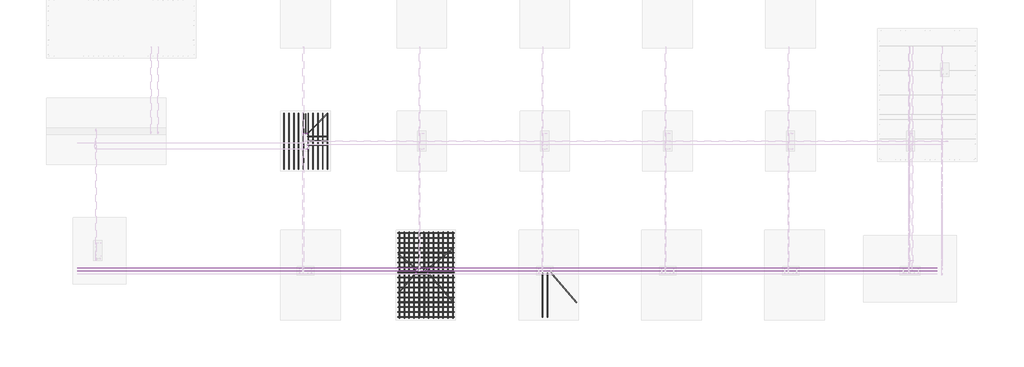
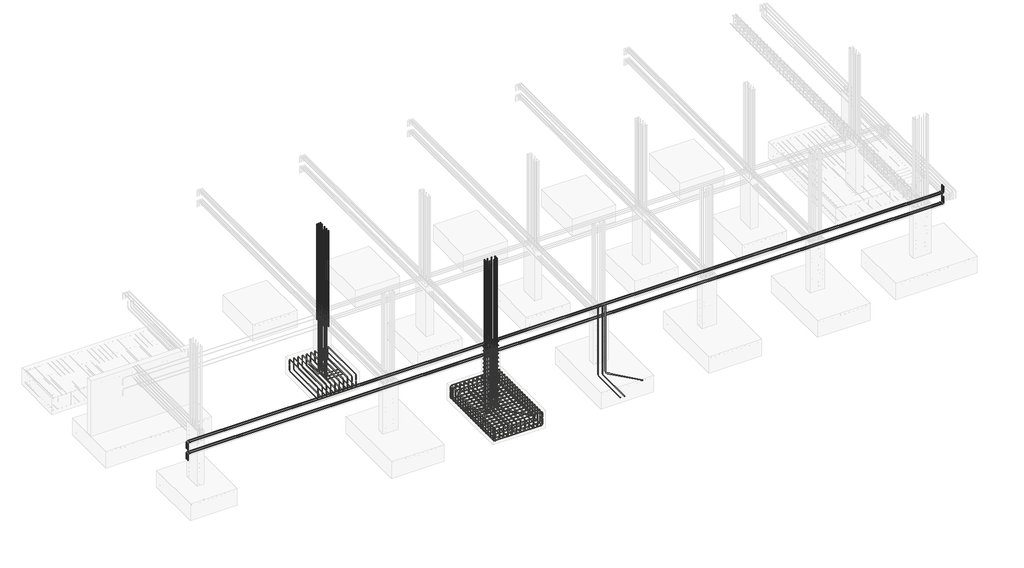
# One storey, part 4 of 18: 38 reinforcing bars.
"""IFC4 building model written with IfcOpenShell, lengths in millimetres."""

from ifc_helpers import new_model, si_unit, point, frame, origin, place, context, project, spatial, polyline, circle_curve, trimmed, segment, composite_curve, source, transform, mapped, element, save
from ifc_brep_helpers import swept_disk

model = new_model("IFC4")

# Units and contexts
model_context = context("Model", 3, world=origin())
ifc_project = project(units=[si_unit("LENGTHUNIT", "METRE", prefix="MILLI")], contexts=[model_context])

# Site, building, storey
site = spatial("IfcSite", under=ifc_project)
building = spatial("IfcBuilding", under=site)
storey = spatial("IfcBuildingStorey", under=building, Elevation=-2000.0)

# Reinforcing bars
placement = place(None, origin())
reinforcing_bar_shape = source(origin(), model_context, "Body", "SolidModel", [
    swept_disk(composite_curve([segment(polyline([(-9318.4091864, -811.9600376, -2322.6684255), (-9318.4091864, -811.9600376, -2470.6684255)]), True, "CONTINUOUS"), segment(trimmed(circle_curve(frame((-9318.4091864, -857.9600376, -2470.6684255), z_axis=(-1.0, 0.0, 0.0), x_axis=(0.0, 46.0, 0.0)), 46.0), [point((-9318.4091864, -811.9600376, -2470.6684255))], [point((-9318.4091864, -857.9600376, -2516.6684255))], True, "CARTESIAN"), True, "CONTINUOUS"), segment(polyline([(-9318.4091864, -857.9600376, -2516.6684255), (-9318.4091864, -2453.9600376, -2516.6684255)]), True, "CONTINUOUS"), segment(trimmed(circle_curve(frame((-9318.4091864, -2453.9600376, -2470.6684255), z_axis=(-1.0, 0.0, 0.0), x_axis=(0.0, 0.0, -46.0)), 46.0), [point((-9318.4091864, -2453.9600376, -2516.6684255))], [point((-9318.4091864, -2499.9600376, -2470.6684255))], True, "CARTESIAN"), True, "CONTINUOUS"), segment(polyline([(-9318.4091864, -2499.9600376, -2470.6684255), (-9318.4091864, -2499.9600376, -2322.6684255)]), True, "CONTINUOUS")], self_intersect=False), 6.0),
])
element("IfcReinforcingBar", 1, at=placement, inside=storey, context=model_context, shape_type="MappedRepresentation", body=[
    mapped(reinforcing_bar_shape, transform((0.0, 0.0, 0.0), x_axis=(1.0, 0.0, 0.0), y_axis=(0.0, 1.0, 0.0), z_axis=(0.0, 0.0, 1.0))),
    mapped(reinforcing_bar_shape, transform((144.8687847, 0.0, 0.0), x_axis=(1.0, 0.0, 0.0), y_axis=(0.0, 1.0, 0.0), z_axis=(0.0, 0.0, 1.0))),
    mapped(reinforcing_bar_shape, transform((289.7375694, 0.0, 0.0), x_axis=(1.0, 0.0, 0.0), y_axis=(0.0, 1.0, 0.0), z_axis=(0.0, 0.0, 1.0))),
    mapped(reinforcing_bar_shape, transform((434.6063541, 0.0, 0.0), x_axis=(1.0, 0.0, 0.0), y_axis=(0.0, 1.0, 0.0), z_axis=(0.0, 0.0, 1.0))),
    mapped(reinforcing_bar_shape, transform((579.4751388, 0.0, 0.0), x_axis=(1.0, 0.0, 0.0), y_axis=(0.0, 1.0, 0.0), z_axis=(0.0, 0.0, 1.0))),
    mapped(reinforcing_bar_shape, transform((724.3439235, 0.0, 0.0), x_axis=(1.0, 0.0, 0.0), y_axis=(0.0, 1.0, 0.0), z_axis=(0.0, 0.0, 1.0))),
    mapped(reinforcing_bar_shape, transform((869.2127082, 0.0, 0.0), x_axis=(1.0, 0.0, 0.0), y_axis=(0.0, 1.0, 0.0), z_axis=(0.0, 0.0, 1.0))),
    mapped(reinforcing_bar_shape, transform((1014.0814929, 0.0, 0.0), x_axis=(1.0, 0.0, 0.0), y_axis=(0.0, 1.0, 0.0), z_axis=(0.0, 0.0, 1.0))),
    mapped(reinforcing_bar_shape, transform((1158.9502776, 0.0, 0.0), x_axis=(1.0, 0.0, 0.0), y_axis=(0.0, 1.0, 0.0), z_axis=(0.0, 0.0, 1.0))),
    mapped(reinforcing_bar_shape, transform((1303.8190623, 0.0, 0.0), x_axis=(1.0, 0.0, 0.0), y_axis=(0.0, 1.0, 0.0), z_axis=(0.0, 0.0, 1.0))),
])
reinforcing_bar_2_shape = source(origin(), model_context, "Body", "SolidModel", [
    swept_disk(composite_curve([segment(polyline([(-8012.6669522, -811.9600376, -2276.6677805), (-8012.6669522, -811.9600376, -2128.6677805)]), True, "CONTINUOUS"), segment(trimmed(circle_curve(frame((-8012.6669522, -857.9600376, -2128.6677805), z_axis=(1.0, 0.0, 0.0), x_axis=(0.0, 46.0, 0.0)), 46.0), [point((-8012.6669522, -811.9600376, -2128.6677805))], [point((-8012.6669522, -857.9600376, -2082.6677805))], True, "CARTESIAN"), True, "CONTINUOUS"), segment(polyline([(-8012.6669522, -857.9600376, -2082.6677805), (-8012.6669522, -2453.9600376, -2082.6677805)]), True, "CONTINUOUS"), segment(trimmed(circle_curve(frame((-8012.6669522, -2453.9600376, -2128.6677805), z_axis=(1.0, 0.0, 0.0), x_axis=(0.0, 0.0, 46.0)), 46.0), [point((-8012.6669522, -2453.9600376, -2082.6677805))], [point((-8012.6669522, -2499.9600376, -2128.6677805))], True, "CARTESIAN"), True, "CONTINUOUS"), segment(polyline([(-8012.6669522, -2499.9600376, -2128.6677805), (-8012.6669522, -2499.9600376, -2276.6677805)]), True, "CONTINUOUS")], self_intersect=False), 6.0),
])
element("IfcReinforcingBar", 2, at=placement, inside=storey, context=model_context, shape_type="MappedRepresentation", body=[
    mapped(reinforcing_bar_2_shape, transform((0.0, 0.0, 0.0), x_axis=(1.0, 0.0, 0.0), y_axis=(0.0, 1.0, 0.0), z_axis=(0.0, 0.0, 1.0))),
    mapped(reinforcing_bar_2_shape, transform((-145.0824705, 0.0, 0.0), x_axis=(1.0, 0.0, 0.0), y_axis=(0.0, 1.0, 0.0), z_axis=(0.0, 0.0, 1.0))),
    mapped(reinforcing_bar_2_shape, transform((-290.1649409, 0.0, 0.0), x_axis=(1.0, 0.0, 0.0), y_axis=(0.0, 1.0, 0.0), z_axis=(0.0, 0.0, 1.0))),
    mapped(reinforcing_bar_2_shape, transform((-435.2474114, 0.0, 0.0), x_axis=(1.0, 0.0, 0.0), y_axis=(0.0, 1.0, 0.0), z_axis=(0.0, 0.0, 1.0))),
    mapped(reinforcing_bar_2_shape, transform((-580.3298819, 0.0, 0.0), x_axis=(1.0, 0.0, 0.0), y_axis=(0.0, 1.0, 0.0), z_axis=(0.0, 0.0, 1.0))),
    mapped(reinforcing_bar_2_shape, transform((-725.4123523, 0.0, 0.0), x_axis=(1.0, 0.0, 0.0), y_axis=(0.0, 1.0, 0.0), z_axis=(0.0, 0.0, 1.0))),
    mapped(reinforcing_bar_2_shape, transform((-870.4948228, 0.0, 0.0), x_axis=(1.0, 0.0, 0.0), y_axis=(0.0, 1.0, 0.0), z_axis=(0.0, 0.0, 1.0))),
    mapped(reinforcing_bar_2_shape, transform((-1015.5772932, 0.0, 0.0), x_axis=(1.0, 0.0, 0.0), y_axis=(0.0, 1.0, 0.0), z_axis=(0.0, 0.0, 1.0))),
    mapped(reinforcing_bar_2_shape, transform((-1160.6597637, 0.0, 0.0), x_axis=(1.0, 0.0, 0.0), y_axis=(0.0, 1.0, 0.0), z_axis=(0.0, 0.0, 1.0))),
    mapped(reinforcing_bar_2_shape, transform((-1305.7422342, 0.0, 0.0), x_axis=(1.0, 0.0, 0.0), y_axis=(0.0, 1.0, 0.0), z_axis=(0.0, 0.0, 1.0))),
])
reinforcing_bar_3_shape = source(origin(), model_context, "Body", "SolidModel", [
    swept_disk(composite_curve([segment(polyline([(-4208.2940057, -4415.5752408, -2300.0), (-4208.2940057, -4415.5752408, -2486.6)]), True, "CONTINUOUS"), segment(trimmed(circle_curve(frame((-4263.7440057, -4415.5752408, -2486.6), z_axis=(0.0, 1.0, 0.0), x_axis=(55.45000000000073, 0.0, 0.0)), 55.45), [point((-4208.2940057, -4415.5752408, -2486.6))], [point((-4263.7440057, -4415.5752408, -2542.05))], True, "CARTESIAN"), True, "CONTINUOUS"), segment(polyline([(-4263.7440057, -4415.5752408, -2542.05), (-5836.9440057, -4415.5752408, -2542.05)]), True, "CONTINUOUS"), segment(trimmed(circle_curve(frame((-5836.9440057, -4415.5752408, -2486.6), z_axis=(0.0, 1.0, 0.0), x_axis=(0.0, 0.0, -55.45000000000027)), 55.45), [point((-5836.9440057, -4415.5752408, -2542.05))], [point((-5892.3940057, -4415.5752408, -2486.6))], True, "CARTESIAN"), True, "CONTINUOUS"), segment(polyline([(-5892.3940057, -4415.5752408, -2486.6), (-5892.3940057, -4415.5752408, -2300.0)]), True, "CONTINUOUS")], self_intersect=False), 7.95),
])
element("IfcReinforcingBar", 3, at=placement, inside=storey, context=model_context, shape_type="MappedRepresentation", body=[
    mapped(reinforcing_bar_3_shape, transform((0.0, 0.0, 0.0), x_axis=(1.0, 0.0, 0.0), y_axis=(0.0, 1.0, 0.0), z_axis=(0.0, 0.0, 1.0))),
    mapped(reinforcing_bar_3_shape, transform((0.0, -148.9809282, 0.0), x_axis=(1.0, 0.0, 0.0), y_axis=(0.0, 1.0, 0.0), z_axis=(0.0, 0.0, 1.0))),
    mapped(reinforcing_bar_3_shape, transform((0.0, -297.9618564, 0.0), x_axis=(1.0, 0.0, 0.0), y_axis=(0.0, 1.0, 0.0), z_axis=(0.0, 0.0, 1.0))),
    mapped(reinforcing_bar_3_shape, transform((0.0, -446.9427846, 0.0), x_axis=(1.0, 0.0, 0.0), y_axis=(0.0, 1.0, 0.0), z_axis=(0.0, 0.0, 1.0))),
    mapped(reinforcing_bar_3_shape, transform((0.0, -595.9237129, 0.0), x_axis=(1.0, 0.0, 0.0), y_axis=(0.0, 1.0, 0.0), z_axis=(0.0, 0.0, 1.0))),
    mapped(reinforcing_bar_3_shape, transform((0.0, -744.9046411, 0.0), x_axis=(1.0, 0.0, 0.0), y_axis=(0.0, 1.0, 0.0), z_axis=(0.0, 0.0, 1.0))),
    mapped(reinforcing_bar_3_shape, transform((0.0, -893.8855693, 0.0), x_axis=(1.0, 0.0, 0.0), y_axis=(0.0, 1.0, 0.0), z_axis=(0.0, 0.0, 1.0))),
    mapped(reinforcing_bar_3_shape, transform((0.0, -1042.8664975, 0.0), x_axis=(1.0, 0.0, 0.0), y_axis=(0.0, 1.0, 0.0), z_axis=(0.0, 0.0, 1.0))),
    mapped(reinforcing_bar_3_shape, transform((0.0, -1191.8474257, 0.0), x_axis=(1.0, 0.0, 0.0), y_axis=(0.0, 1.0, 0.0), z_axis=(0.0, 0.0, 1.0))),
    mapped(reinforcing_bar_3_shape, transform((0.0, -1340.8283539, 0.0), x_axis=(1.0, 0.0, 0.0), y_axis=(0.0, 1.0, 0.0), z_axis=(0.0, 0.0, 1.0))),
    mapped(reinforcing_bar_3_shape, transform((0.0, -1489.8092821, 0.0), x_axis=(1.0, 0.0, 0.0), y_axis=(0.0, 1.0, 0.0), z_axis=(0.0, 0.0, 1.0))),
    mapped(reinforcing_bar_3_shape, transform((0.0, -1638.7902103, 0.0), x_axis=(1.0, 0.0, 0.0), y_axis=(0.0, 1.0, 0.0), z_axis=(0.0, 0.0, 1.0))),
    mapped(reinforcing_bar_3_shape, transform((0.0, -1787.7711386, 0.0), x_axis=(1.0, 0.0, 0.0), y_axis=(0.0, 1.0, 0.0), z_axis=(0.0, 0.0, 1.0))),
    mapped(reinforcing_bar_3_shape, transform((0.0, -1936.7520668, 0.0), x_axis=(1.0, 0.0, 0.0), y_axis=(0.0, 1.0, 0.0), z_axis=(0.0, 0.0, 1.0))),
    mapped(reinforcing_bar_3_shape, transform((0.0, -2085.732995, 0.0), x_axis=(1.0, 0.0, 0.0), y_axis=(0.0, 1.0, 0.0), z_axis=(0.0, 0.0, 1.0))),
    mapped(reinforcing_bar_3_shape, transform((0.0, -2234.7139232, 0.0), x_axis=(1.0, 0.0, 0.0), y_axis=(0.0, 1.0, 0.0), z_axis=(0.0, 0.0, 1.0))),
    mapped(reinforcing_bar_3_shape, transform((0.0, -2383.6948514, 0.0), x_axis=(1.0, 0.0, 0.0), y_axis=(0.0, 1.0, 0.0), z_axis=(0.0, 0.0, 1.0))),
    mapped(reinforcing_bar_3_shape, transform((0.0, -2532.6757796, 0.0), x_axis=(1.0, 0.0, 0.0), y_axis=(0.0, 1.0, 0.0), z_axis=(0.0, 0.0, 1.0))),
])
reinforcing_bar_4_shape = source(origin(), model_context, "Body", "SolidModel", [
    swept_disk(composite_curve([segment(polyline([(-5894.3440057, -4415.5752408, -2250.0), (-5894.3440057, -4415.5752408, -2102.0)]), True, "CONTINUOUS"), segment(trimmed(circle_curve(frame((-5848.3440057, -4415.5752408, -2102.0), z_axis=(0.0, 1.0, 0.0), x_axis=(-46.0, 0.0, 0.0)), 46.0), [point((-5894.3440057, -4415.5752408, -2102.0))], [point((-5848.3440057, -4415.5752408, -2056.0))], True, "CARTESIAN"), True, "CONTINUOUS"), segment(polyline([(-5848.3440057, -4415.5752408, -2056.0), (-4252.3440057, -4415.5752408, -2056.0)]), True, "CONTINUOUS"), segment(trimmed(circle_curve(frame((-4252.3440057, -4415.5752408, -2102.0), z_axis=(0.0, 1.0, 0.0), x_axis=(0.0, 0.0, 46.0)), 46.0), [point((-4252.3440057, -4415.5752408, -2056.0))], [point((-4206.3440057, -4415.5752408, -2102.0))], True, "CARTESIAN"), True, "CONTINUOUS"), segment(polyline([(-4206.3440057, -4415.5752408, -2102.0), (-4206.3440057, -4415.5752408, -2250.0)]), True, "CONTINUOUS")], self_intersect=False), 6.0),
])
element("IfcReinforcingBar", 4, at=placement, inside=storey, context=model_context, shape_type="MappedRepresentation", body=[
    mapped(reinforcing_bar_4_shape, transform((0.0, 0.0, 0.0), x_axis=(1.0, 0.0, 0.0), y_axis=(0.0, 1.0, 0.0), z_axis=(0.0, 0.0, 1.0))),
    mapped(reinforcing_bar_4_shape, transform((0.0, -148.9809282, 0.0), x_axis=(1.0, 0.0, 0.0), y_axis=(0.0, 1.0, 0.0), z_axis=(0.0, 0.0, 1.0))),
    mapped(reinforcing_bar_4_shape, transform((0.0, -297.9618564, 0.0), x_axis=(1.0, 0.0, 0.0), y_axis=(0.0, 1.0, 0.0), z_axis=(0.0, 0.0, 1.0))),
    mapped(reinforcing_bar_4_shape, transform((0.0, -446.9427846, 0.0), x_axis=(1.0, 0.0, 0.0), y_axis=(0.0, 1.0, 0.0), z_axis=(0.0, 0.0, 1.0))),
    mapped(reinforcing_bar_4_shape, transform((0.0, -595.9237129, 0.0), x_axis=(1.0, 0.0, 0.0), y_axis=(0.0, 1.0, 0.0), z_axis=(0.0, 0.0, 1.0))),
    mapped(reinforcing_bar_4_shape, transform((0.0, -744.9046411, 0.0), x_axis=(1.0, 0.0, 0.0), y_axis=(0.0, 1.0, 0.0), z_axis=(0.0, 0.0, 1.0))),
    mapped(reinforcing_bar_4_shape, transform((0.0, -893.8855693, 0.0), x_axis=(1.0, 0.0, 0.0), y_axis=(0.0, 1.0, 0.0), z_axis=(0.0, 0.0, 1.0))),
    mapped(reinforcing_bar_4_shape, transform((0.0, -1042.8664975, 0.0), x_axis=(1.0, 0.0, 0.0), y_axis=(0.0, 1.0, 0.0), z_axis=(0.0, 0.0, 1.0))),
    mapped(reinforcing_bar_4_shape, transform((0.0, -1191.8474257, 0.0), x_axis=(1.0, 0.0, 0.0), y_axis=(0.0, 1.0, 0.0), z_axis=(0.0, 0.0, 1.0))),
    mapped(reinforcing_bar_4_shape, transform((0.0, -1340.8283539, 0.0), x_axis=(1.0, 0.0, 0.0), y_axis=(0.0, 1.0, 0.0), z_axis=(0.0, 0.0, 1.0))),
    mapped(reinforcing_bar_4_shape, transform((0.0, -1489.8092821, 0.0), x_axis=(1.0, 0.0, 0.0), y_axis=(0.0, 1.0, 0.0), z_axis=(0.0, 0.0, 1.0))),
    mapped(reinforcing_bar_4_shape, transform((0.0, -1638.7902103, 0.0), x_axis=(1.0, 0.0, 0.0), y_axis=(0.0, 1.0, 0.0), z_axis=(0.0, 0.0, 1.0))),
    mapped(reinforcing_bar_4_shape, transform((0.0, -1787.7711386, 0.0), x_axis=(1.0, 0.0, 0.0), y_axis=(0.0, 1.0, 0.0), z_axis=(0.0, 0.0, 1.0))),
    mapped(reinforcing_bar_4_shape, transform((0.0, -1936.7520668, 0.0), x_axis=(1.0, 0.0, 0.0), y_axis=(0.0, 1.0, 0.0), z_axis=(0.0, 0.0, 1.0))),
    mapped(reinforcing_bar_4_shape, transform((0.0, -2085.732995, 0.0), x_axis=(1.0, 0.0, 0.0), y_axis=(0.0, 1.0, 0.0), z_axis=(0.0, 0.0, 1.0))),
    mapped(reinforcing_bar_4_shape, transform((0.0, -2234.7139232, 0.0), x_axis=(1.0, 0.0, 0.0), y_axis=(0.0, 1.0, 0.0), z_axis=(0.0, 0.0, 1.0))),
    mapped(reinforcing_bar_4_shape, transform((0.0, -2383.6948514, 0.0), x_axis=(1.0, 0.0, 0.0), y_axis=(0.0, 1.0, 0.0), z_axis=(0.0, 0.0, 1.0))),
    mapped(reinforcing_bar_4_shape, transform((0.0, -2532.6757796, 0.0), x_axis=(1.0, 0.0, 0.0), y_axis=(0.0, 1.0, 0.0), z_axis=(0.0, 0.0, 1.0))),
])
reinforcing_bar_5_shape = source(origin(), model_context, "Body", "SolidModel", [
    swept_disk(composite_curve([segment(polyline([(-5848.1632229, -4392.6797656, -2322.6684255), (-5848.1632229, -4392.6797656, -2470.6684255)]), True, "CONTINUOUS"), segment(trimmed(circle_curve(frame((-5848.1632229, -4438.6797656, -2470.6684255), z_axis=(-1.0, 0.0, 0.0), x_axis=(0.0, 46.0, 0.0)), 46.0), [point((-5848.1632229, -4392.6797656, -2470.6684255))], [point((-5848.1632229, -4438.6797656, -2516.6684255))], True, "CARTESIAN"), True, "CONTINUOUS"), segment(polyline([(-5848.1632229, -4438.6797656, -2516.6684255), (-5848.1632229, -6934.6797656, -2516.6684255)]), True, "CONTINUOUS"), segment(trimmed(circle_curve(frame((-5848.1632229, -6934.6797656, -2470.6684255), z_axis=(-1.0, 0.0, 0.0), x_axis=(0.0, 0.0, -46.0)), 46.0), [point((-5848.1632229, -6934.6797656, -2516.6684255))], [point((-5848.1632229, -6980.6797656, -2470.6684255))], True, "CARTESIAN"), True, "CONTINUOUS"), segment(polyline([(-5848.1632229, -6980.6797656, -2470.6684255), (-5848.1632229, -6980.6797656, -2322.6684255)]), True, "CONTINUOUS")], self_intersect=False), 6.0),
])
element("IfcReinforcingBar", 5, at=placement, inside=storey, context=model_context, shape_type="MappedRepresentation", body=[
    mapped(reinforcing_bar_5_shape, transform((0.0, 0.0, 0.0), x_axis=(1.0, 0.0, 0.0), y_axis=(0.0, 1.0, 0.0), z_axis=(0.0, 0.0, 1.0))),
    mapped(reinforcing_bar_5_shape, transform((145.8017329, 0.0, 0.0), x_axis=(1.0, 0.0, 0.0), y_axis=(0.0, 1.0, 0.0), z_axis=(0.0, 0.0, 1.0))),
    mapped(reinforcing_bar_5_shape, transform((291.6034659, 0.0, 0.0), x_axis=(1.0, 0.0, 0.0), y_axis=(0.0, 1.0, 0.0), z_axis=(0.0, 0.0, 1.0))),
    mapped(reinforcing_bar_5_shape, transform((437.4051988, 0.0, 0.0), x_axis=(1.0, 0.0, 0.0), y_axis=(0.0, 1.0, 0.0), z_axis=(0.0, 0.0, 1.0))),
    mapped(reinforcing_bar_5_shape, transform((583.2069318, 0.0, 0.0), x_axis=(1.0, 0.0, 0.0), y_axis=(0.0, 1.0, 0.0), z_axis=(0.0, 0.0, 1.0))),
    mapped(reinforcing_bar_5_shape, transform((729.0086647, 0.0, 0.0), x_axis=(1.0, 0.0, 0.0), y_axis=(0.0, 1.0, 0.0), z_axis=(0.0, 0.0, 1.0))),
    mapped(reinforcing_bar_5_shape, transform((874.8103976, 0.0, 0.0), x_axis=(1.0, 0.0, 0.0), y_axis=(0.0, 1.0, 0.0), z_axis=(0.0, 0.0, 1.0))),
    mapped(reinforcing_bar_5_shape, transform((1020.6121306, 0.0, 0.0), x_axis=(1.0, 0.0, 0.0), y_axis=(0.0, 1.0, 0.0), z_axis=(0.0, 0.0, 1.0))),
    mapped(reinforcing_bar_5_shape, transform((1166.4138635, 0.0, 0.0), x_axis=(1.0, 0.0, 0.0), y_axis=(0.0, 1.0, 0.0), z_axis=(0.0, 0.0, 1.0))),
    mapped(reinforcing_bar_5_shape, transform((1312.2155965, 0.0, 0.0), x_axis=(1.0, 0.0, 0.0), y_axis=(0.0, 1.0, 0.0), z_axis=(0.0, 0.0, 1.0))),
    mapped(reinforcing_bar_5_shape, transform((1458.0173294, 0.0, 0.0), x_axis=(1.0, 0.0, 0.0), y_axis=(0.0, 1.0, 0.0), z_axis=(0.0, 0.0, 1.0))),
    mapped(reinforcing_bar_5_shape, transform((1603.8190623, 0.0, 0.0), x_axis=(1.0, 0.0, 0.0), y_axis=(0.0, 1.0, 0.0), z_axis=(0.0, 0.0, 1.0))),
])
reinforcing_bar_6_shape = source(origin(), model_context, "Body", "SolidModel", [
    swept_disk(composite_curve([segment(polyline([(-4242.4209887, -4392.6797656, -2276.6677805), (-4242.4209887, -4392.6797656, -2128.6677805)]), True, "CONTINUOUS"), segment(trimmed(circle_curve(frame((-4242.4209887, -4438.6797656, -2128.6677805), z_axis=(1.0, 0.0, 0.0), x_axis=(0.0, 46.0, 0.0)), 46.0), [point((-4242.4209887, -4392.6797656, -2128.6677805))], [point((-4242.4209887, -4438.6797656, -2082.6677805))], True, "CARTESIAN"), True, "CONTINUOUS"), segment(polyline([(-4242.4209887, -4438.6797656, -2082.6677805), (-4242.4209887, -6934.6797656, -2082.6677805)]), True, "CONTINUOUS"), segment(trimmed(circle_curve(frame((-4242.4209887, -6934.6797656, -2128.6677805), z_axis=(1.0, 0.0, 0.0), x_axis=(0.0, 0.0, 46.0)), 46.0), [point((-4242.4209887, -6934.6797656, -2082.6677805))], [point((-4242.4209887, -6980.6797656, -2128.6677805))], True, "CARTESIAN"), True, "CONTINUOUS"), segment(polyline([(-4242.4209887, -6980.6797656, -2128.6677805), (-4242.4209887, -6980.6797656, -2276.6677805)]), True, "CONTINUOUS")], self_intersect=False), 6.0),
])
element("IfcReinforcingBar", 6, at=placement, inside=storey, context=model_context, shape_type="MappedRepresentation", body=[
    mapped(reinforcing_bar_6_shape, transform((0.0, 0.0, 0.0), x_axis=(1.0, 0.0, 0.0), y_axis=(0.0, 1.0, 0.0), z_axis=(0.0, 0.0, 1.0))),
    mapped(reinforcing_bar_6_shape, transform((-145.9765667, 0.0, 0.0), x_axis=(1.0, 0.0, 0.0), y_axis=(0.0, 1.0, 0.0), z_axis=(0.0, 0.0, 1.0))),
    mapped(reinforcing_bar_6_shape, transform((-291.9531335, 0.0, 0.0), x_axis=(1.0, 0.0, 0.0), y_axis=(0.0, 1.0, 0.0), z_axis=(0.0, 0.0, 1.0))),
    mapped(reinforcing_bar_6_shape, transform((-437.9297002, 0.0, 0.0), x_axis=(1.0, 0.0, 0.0), y_axis=(0.0, 1.0, 0.0), z_axis=(0.0, 0.0, 1.0))),
    mapped(reinforcing_bar_6_shape, transform((-583.906267, 0.0, 0.0), x_axis=(1.0, 0.0, 0.0), y_axis=(0.0, 1.0, 0.0), z_axis=(0.0, 0.0, 1.0))),
    mapped(reinforcing_bar_6_shape, transform((-729.8828337, 0.0, 0.0), x_axis=(1.0, 0.0, 0.0), y_axis=(0.0, 1.0, 0.0), z_axis=(0.0, 0.0, 1.0))),
    mapped(reinforcing_bar_6_shape, transform((-875.8594005, 0.0, 0.0), x_axis=(1.0, 0.0, 0.0), y_axis=(0.0, 1.0, 0.0), z_axis=(0.0, 0.0, 1.0))),
    mapped(reinforcing_bar_6_shape, transform((-1021.8359672, 0.0, 0.0), x_axis=(1.0, 0.0, 0.0), y_axis=(0.0, 1.0, 0.0), z_axis=(0.0, 0.0, 1.0))),
    mapped(reinforcing_bar_6_shape, transform((-1167.8125339, 0.0, 0.0), x_axis=(1.0, 0.0, 0.0), y_axis=(0.0, 1.0, 0.0), z_axis=(0.0, 0.0, 1.0))),
    mapped(reinforcing_bar_6_shape, transform((-1313.7891007, 0.0, 0.0), x_axis=(1.0, 0.0, 0.0), y_axis=(0.0, 1.0, 0.0), z_axis=(0.0, 0.0, 1.0))),
    mapped(reinforcing_bar_6_shape, transform((-1459.7656674, 0.0, 0.0), x_axis=(1.0, 0.0, 0.0), y_axis=(0.0, 1.0, 0.0), z_axis=(0.0, 0.0, 1.0))),
    mapped(reinforcing_bar_6_shape, transform((-1605.7422342, 0.0, 0.0), x_axis=(1.0, 0.0, 0.0), y_axis=(0.0, 1.0, 0.0), z_axis=(0.0, 0.0, 1.0))),
])
element("IfcReinforcingBar", 7, at=placement, inside=storey, context=model_context, shape_type="SolidModel", body=[
    swept_disk(composite_curve([segment(polyline([(-520.063822, -6507.758358, -2480.0), (-1248.148149, -5670.1931504, -2480.0)]), True, "CONTINUOUS"), segment(trimmed(circle_curve(frame((-1248.148149, -5670.1931504, -2412.5), z_axis=(0.7547095802227678, 0.6560590289905122, 0.0), x_axis=(0.0, 0.0, -67.5)), 67.5), [point((-1248.148149, -5670.1931504, -2480.0))], [point((-1292.4321335, -5619.2502537, -2412.5))], True, "CARTESIAN"), True, "CONTINUOUS"), segment(polyline([(-1292.4321335, -5619.2502537, -2412.5), (-1292.4321335, -5619.2502537, -20.0)]), True, "CONTINUOUS")], self_intersect=False), 10.0),
])
reinforcing_bar_7_shape = source(origin(), model_context, "Body", "SolidModel", [
    swept_disk(composite_curve([segment(polyline([(-1543.6420643, -6948.2510204, -2480.0), (-1543.6420643, -5673.717598, -2480.0)]), True, "CONTINUOUS"), segment(trimmed(circle_curve(frame((-1543.6420643, -5673.717598, -2434.0), z_axis=(1.0, 0.0, 0.0), x_axis=(0.0, 0.0, -46.0)), 46.0), [point((-1543.6420643, -5673.717598, -2480.0))], [point((-1543.6420643, -5627.717598, -2434.0))], True, "CARTESIAN"), True, "CONTINUOUS"), segment(polyline([(-1543.6420643, -5627.717598, -2434.0), (-1543.6420643, -5627.717598, -30.0)]), True, "CONTINUOUS")], self_intersect=False), 6.0),
])
element("IfcReinforcingBar", 8, at=placement, inside=storey, context=model_context, shape_type="MappedRepresentation", body=[
    mapped(reinforcing_bar_7_shape, transform((0.0, 0.0, 0.0), x_axis=(1.0, 0.0, 0.0), y_axis=(0.0, 1.0, 0.0), z_axis=(0.0, 0.0, 1.0))),
    mapped(reinforcing_bar_7_shape, transform((144.9594019, 0.0, 0.0), x_axis=(1.0, 0.0, 0.0), y_axis=(0.0, 1.0, 0.0), z_axis=(0.0, 0.0, 1.0))),
])
reinforcing_bar_8_shape = source(origin(), model_context, "Body", "SolidModel", [
    swept_disk(composite_curve([segment(polyline([(-5060.4315175, -5535.5091206, -34.0), (-5004.0960659, -5479.1736689, -34.0)]), True, "CONTINUOUS"), segment(trimmed(circle_curve(frame((-4983.5899692, -5499.6797656, -34.0), z_axis=(0.0, 0.0, -1.0), x_axis=(-20.506096699999944, 20.506096699999944, 0.0)), 29.0), [point((-5004.0960659, -5479.1736689, -34.0))], [point((-4954.5899692, -5499.6797656, -34.0))], True, "CARTESIAN"), True, "CONTINUOUS"), segment(polyline([(-4954.5899692, -5499.6797656, -34.0), (-4954.5899692, -5623.6797656, -34.0)]), True, "CONTINUOUS"), segment(trimmed(circle_curve(frame((-4983.5899692, -5623.6797656, -34.0), z_axis=(0.0, 0.0, -1.0), x_axis=(29.0, 0.0, 0.0)), 29.0), [point((-4954.5899692, -5623.6797656, -34.0))], [point((-4983.5899692, -5652.6797656, -34.0))], True, "CARTESIAN"), True, "CONTINUOUS"), segment(polyline([(-4983.5899692, -5652.6797656, -34.0), (-5357.5899692, -5652.6797656, -34.0)]), True, "CONTINUOUS"), segment(trimmed(circle_curve(frame((-5357.5899692, -5623.707741, -32.7265044), z_axis=(0.0, 0.043913640913297095, -0.9990353307775146), x_axis=(0.0, -28.972024599999713, -1.2734955999999968)), 29.0), [point((-5357.5899692, -5652.6797656, -34.0))], [point((-5386.5899692, -5623.707741, -32.7265044))], True, "CARTESIAN"), True, "CONTINUOUS"), segment(polyline([(-5386.5899692, -5623.707741, -32.7265044), (-5386.5899692, -5499.6517902, -27.2734956)]), True, "CONTINUOUS"), segment(trimmed(circle_curve(frame((-5357.5899692, -5499.6517902, -27.2734956), z_axis=(0.0, 0.043913640913297095, -0.9990353307775146), x_axis=(-29.0, 0.0, 0.0)), 29.0), [point((-5386.5899692, -5499.6517902, -27.2734956))], [point((-5357.5899692, -5470.6797656, -26.0))], True, "CARTESIAN"), True, "CONTINUOUS"), segment(polyline([(-5357.5899692, -5470.6797656, -26.0), (-4983.5899692, -5470.6797656, -26.0)]), True, "CONTINUOUS"), segment(trimmed(circle_curve(frame((-4983.5899692, -5499.6797656, -26.0), z_axis=(0.0, 0.0, -1.0), x_axis=(0.0, 29.0, 0.0)), 29.0), [point((-4983.5899692, -5470.6797656, -26.0))], [point((-4963.0838726, -5520.1858622, -26.0))], True, "CARTESIAN"), True, "CONTINUOUS"), segment(polyline([(-4963.0838726, -5520.1858622, -26.0), (-5019.4193242, -5576.5213139, -26.0)]), True, "CONTINUOUS")], self_intersect=False), 4.0),
])
element("IfcReinforcingBar", 9, at=placement, inside=storey, context=model_context, shape_type="MappedRepresentation", body=[
    mapped(reinforcing_bar_8_shape, transform((0.0, 0.0, 0.0), x_axis=(1.0, 0.0, 0.0), y_axis=(0.0, 1.0, 0.0), z_axis=(0.0, 0.0, 1.0))),
    mapped(reinforcing_bar_8_shape, transform((0.0, 0.0, -148.6153846), x_axis=(1.0, 0.0, 0.0), y_axis=(0.0, 1.0, 0.0), z_axis=(0.0, 0.0, 1.0))),
    mapped(reinforcing_bar_8_shape, transform((0.0, 0.0, -297.2307692), x_axis=(1.0, 0.0, 0.0), y_axis=(0.0, 1.0, 0.0), z_axis=(0.0, 0.0, 1.0))),
    mapped(reinforcing_bar_8_shape, transform((0.0, 0.0, -445.8461538), x_axis=(1.0, 0.0, 0.0), y_axis=(0.0, 1.0, 0.0), z_axis=(0.0, 0.0, 1.0))),
    mapped(reinforcing_bar_8_shape, transform((0.0, 0.0, -594.4615385), x_axis=(1.0, 0.0, 0.0), y_axis=(0.0, 1.0, 0.0), z_axis=(0.0, 0.0, 1.0))),
    mapped(reinforcing_bar_8_shape, transform((0.0, 0.0, -743.0769231), x_axis=(1.0, 0.0, 0.0), y_axis=(0.0, 1.0, 0.0), z_axis=(0.0, 0.0, 1.0))),
    mapped(reinforcing_bar_8_shape, transform((0.0, 0.0, -891.6923077), x_axis=(1.0, 0.0, 0.0), y_axis=(0.0, 1.0, 0.0), z_axis=(0.0, 0.0, 1.0))),
    mapped(reinforcing_bar_8_shape, transform((0.0, 0.0, -1040.3076923), x_axis=(1.0, 0.0, 0.0), y_axis=(0.0, 1.0, 0.0), z_axis=(0.0, 0.0, 1.0))),
    mapped(reinforcing_bar_8_shape, transform((0.0, 0.0, -1188.9230769), x_axis=(1.0, 0.0, 0.0), y_axis=(0.0, 1.0, 0.0), z_axis=(0.0, 0.0, 1.0))),
    mapped(reinforcing_bar_8_shape, transform((0.0, 0.0, -1337.5384615), x_axis=(1.0, 0.0, 0.0), y_axis=(0.0, 1.0, 0.0), z_axis=(0.0, 0.0, 1.0))),
    mapped(reinforcing_bar_8_shape, transform((0.0, 0.0, -1486.1538462), x_axis=(1.0, 0.0, 0.0), y_axis=(0.0, 1.0, 0.0), z_axis=(0.0, 0.0, 1.0))),
    mapped(reinforcing_bar_8_shape, transform((0.0, 0.0, -1634.7692308), x_axis=(1.0, 0.0, 0.0), y_axis=(0.0, 1.0, 0.0), z_axis=(0.0, 0.0, 1.0))),
    mapped(reinforcing_bar_8_shape, transform((0.0, 0.0, -1783.3846154), x_axis=(1.0, 0.0, 0.0), y_axis=(0.0, 1.0, 0.0), z_axis=(0.0, 0.0, 1.0))),
    mapped(reinforcing_bar_8_shape, transform((0.0, 0.0, -1932.0), x_axis=(1.0, 0.0, 0.0), y_axis=(0.0, 1.0, 0.0), z_axis=(0.0, 0.0, 1.0))),
])
element("IfcReinforcingBar", 10, at=placement, inside=storey, context=model_context, shape_type="SolidModel", body=[
    swept_disk(composite_curve([segment(polyline([(-5873.6233428, -5063.6864072, -2480.0), (-5400.4558049, -5460.7211138, -2480.0)]), True, "CONTINUOUS"), segment(trimmed(circle_curve(frame((-5400.4558049, -5460.7211138, -2412.5), z_axis=(-0.6427876096865429, -0.766044443118975, 0.0), x_axis=(0.0, 0.0, -67.5)), 67.5), [point((-5400.4558049, -5460.7211138, -2480.0))], [point((-5348.747805, -5504.1092774, -2412.5))], True, "CARTESIAN"), True, "CONTINUOUS"), segment(polyline([(-5348.747805, -5504.1092774, -2412.5), (-5348.747805, -5504.1092774, -20.0)]), True, "CONTINUOUS")], self_intersect=False), 10.0),
])
element("IfcReinforcingBar", 11, at=placement, inside=storey, context=model_context, shape_type="SolidModel", body=[
    swept_disk(composite_curve([segment(polyline([(-5877.6576621, -5559.3632831, -2480.0), (-5405.107931, -5559.3632831, -2480.0)]), True, "CONTINUOUS"), segment(trimmed(circle_curve(frame((-5405.107931, -5559.3632831, -2434.0), z_axis=(0.0, -1.0, 0.0), x_axis=(0.0, 0.0, -46.0)), 46.0), [point((-5405.107931, -5559.3632831, -2480.0))], [point((-5359.107931, -5559.3632831, -2434.0))], True, "CARTESIAN"), True, "CONTINUOUS"), segment(polyline([(-5359.107931, -5559.3632831, -2434.0), (-5359.107931, -5559.3632831, -30.0)]), True, "CONTINUOUS")], self_intersect=False), 6.0),
])
element("IfcReinforcingBar", 12, at=placement, inside=storey, context=model_context, shape_type="SolidModel", body=[
    swept_disk(composite_curve([segment(polyline([(-4227.0646685, -4861.8897199, -2480.0), (-4940.7241336, -5460.7211138, -2480.0)]), True, "CONTINUOUS"), segment(trimmed(circle_curve(frame((-4940.7241336, -5460.7211138, -2412.5), z_axis=(-0.6427876096865429, 0.766044443118975, 0.0), x_axis=(0.0, 0.0, -67.5)), 67.5), [point((-4940.7241336, -5460.7211138, -2480.0))], [point((-4992.4321335, -5504.1092774, -2412.5))], True, "CARTESIAN"), True, "CONTINUOUS"), segment(polyline([(-4992.4321335, -5504.1092774, -2412.5), (-4992.4321335, -5504.1092774, -20.0)]), True, "CONTINUOUS")], self_intersect=False), 10.0),
])
element("IfcReinforcingBar", 13, at=placement, inside=storey, context=model_context, shape_type="SolidModel", body=[
    swept_disk(composite_curve([segment(polyline([(-5880.6241894, -6231.1040429, -2480.0), (-5393.0317894, -5670.1931504, -2480.0)]), True, "CONTINUOUS"), segment(trimmed(circle_curve(frame((-5393.0317894, -5670.1931504, -2412.5), z_axis=(0.7547095802227678, -0.6560590289905122, 0.0), x_axis=(0.0, 0.0, -67.5)), 67.5), [point((-5393.0317894, -5670.1931504, -2480.0))], [point((-5348.747805, -5619.2502537, -2412.5))], True, "CARTESIAN"), True, "CONTINUOUS"), segment(polyline([(-5348.747805, -5619.2502537, -2412.5), (-5348.747805, -5619.2502537, -20.0)]), True, "CONTINUOUS")], self_intersect=False), 10.0),
])
element("IfcReinforcingBar", 14, at=placement, inside=storey, context=model_context, shape_type="SolidModel", body=[
    swept_disk(composite_curve([segment(polyline([(-4220.063822, -6507.758358, -2480.0), (-4948.148149, -5670.1931504, -2480.0)]), True, "CONTINUOUS"), segment(trimmed(circle_curve(frame((-4948.148149, -5670.1931504, -2412.5), z_axis=(0.7547095802227678, 0.6560590289905122, 0.0), x_axis=(0.0, 0.0, -67.5)), 67.5), [point((-4948.148149, -5670.1931504, -2480.0))], [point((-4992.4321335, -5619.2502537, -2412.5))], True, "CARTESIAN"), True, "CONTINUOUS"), segment(polyline([(-4992.4321335, -5619.2502537, -2412.5), (-4992.4321335, -5619.2502537, -20.0)]), True, "CONTINUOUS")], self_intersect=False), 10.0),
])
element("IfcReinforcingBar", 15, at=placement, inside=storey, context=model_context, shape_type="SolidModel", body=[
    swept_disk(composite_curve([segment(polyline([(-4223.0303493, -5559.3632831, -2480.0), (-4936.0720074, -5559.3632831, -2480.0)]), True, "CONTINUOUS"), segment(trimmed(circle_curve(frame((-4936.0720074, -5559.3632831, -2434.0), z_axis=(0.0, 1.0, 0.0), x_axis=(0.0, 0.0, -46.0)), 46.0), [point((-4936.0720074, -5559.3632831, -2480.0))], [point((-4982.0720074, -5559.3632831, -2434.0))], True, "CARTESIAN"), True, "CONTINUOUS"), segment(polyline([(-4982.0720074, -5559.3632831, -2434.0), (-4982.0720074, -5559.3632831, -30.0)]), True, "CONTINUOUS")], self_intersect=False), 6.0),
])
reinforcing_bar_9_shape = source(origin(), model_context, "Body", "SolidModel", [
    swept_disk(composite_curve([segment(polyline([(-5243.6420643, -6948.2510204, -2480.0), (-5243.6420643, -5673.717598, -2480.0)]), True, "CONTINUOUS"), segment(trimmed(circle_curve(frame((-5243.6420643, -5673.717598, -2434.0), z_axis=(1.0, 0.0, 0.0), x_axis=(0.0, 0.0, -46.0)), 46.0), [point((-5243.6420643, -5673.717598, -2480.0))], [point((-5243.6420643, -5627.717598, -2434.0))], True, "CARTESIAN"), True, "CONTINUOUS"), segment(polyline([(-5243.6420643, -5627.717598, -2434.0), (-5243.6420643, -5627.717598, -30.0)]), True, "CONTINUOUS")], self_intersect=False), 6.0),
])
element("IfcReinforcingBar", 16, at=placement, inside=storey, context=model_context, shape_type="MappedRepresentation", body=[
    mapped(reinforcing_bar_9_shape, transform((0.0, 0.0, 0.0), x_axis=(1.0, 0.0, 0.0), y_axis=(0.0, 1.0, 0.0), z_axis=(0.0, 0.0, 1.0))),
    mapped(reinforcing_bar_9_shape, transform((144.9594019, 0.0, 0.0), x_axis=(1.0, 0.0, 0.0), y_axis=(0.0, 1.0, 0.0), z_axis=(0.0, 0.0, 1.0))),
])
reinforcing_bar_10_shape = source(origin(), model_context, "Body", "SolidModel", [
    swept_disk(composite_curve([segment(polyline([(-5243.6420643, -4416.634351, -2480.0), (-5243.6420643, -5449.6419331, -2480.0)]), True, "CONTINUOUS"), segment(trimmed(circle_curve(frame((-5243.6420643, -5449.6419331, -2434.0), z_axis=(-1.0, 0.0, 0.0), x_axis=(0.0, 0.0, -46.0)), 46.0), [point((-5243.6420643, -5449.6419331, -2480.0))], [point((-5243.6420643, -5495.6419331, -2434.0))], True, "CARTESIAN"), True, "CONTINUOUS"), segment(polyline([(-5243.6420643, -5495.6419331, -2434.0), (-5243.6420643, -5495.6419331, -30.0)]), True, "CONTINUOUS")], self_intersect=False), 6.0),
])
element("IfcReinforcingBar", 17, at=placement, inside=storey, context=model_context, shape_type="MappedRepresentation", body=[
    mapped(reinforcing_bar_10_shape, transform((0.0, 0.0, 0.0), x_axis=(1.0, 0.0, 0.0), y_axis=(0.0, 1.0, 0.0), z_axis=(0.0, 0.0, 1.0))),
    mapped(reinforcing_bar_10_shape, transform((144.9594019, 0.0, 0.0), x_axis=(1.0, 0.0, 0.0), y_axis=(0.0, 1.0, 0.0), z_axis=(0.0, 0.0, 1.0))),
])
element("IfcReinforcingBar", 18, at=placement, inside=storey, context=model_context, shape_type="SolidModel", body=[
    swept_disk(composite_curve([segment(polyline([(-8671.037887, -1418.4824597, -30.0), (-8671.037887, -1418.4824597, -2440.6)]), True, "CONTINUOUS"), segment(trimmed(circle_curve(frame((-8671.037887, -1372.4824597, -2440.6), z_axis=(1.0, 0.0, 0.0), x_axis=(0.0, -46.0, 0.0)), 46.0), [point((-8671.037887, -1418.4824597, -2440.6))], [point((-8671.037887, -1372.4824597, -2486.6))], True, "CARTESIAN"), True, "CONTINUOUS"), segment(polyline([(-8671.037887, -1372.4824597, -2486.6), (-8671.037887, -834.8555128, -2486.6)]), True, "CONTINUOUS")], self_intersect=False), 6.0),
])
reinforcing_bar_11_shape = source(origin(), model_context, "Body", "SolidModel", [
    swept_disk(composite_curve([segment(polyline([(-8606.6833135, -1776.5422299, -30.0), (-8606.6833135, -1776.5422299, -2436.6982733)]), True, "CONTINUOUS"), segment(trimmed(circle_curve(frame((-8560.6833135, -1776.5422299, -2436.6982733), z_axis=(0.0, -1.0, 0.0), x_axis=(-46.0, 0.0, 0.0)), 46.0), [point((-8606.6833135, -1776.5422299, -2436.6982733))], [point((-8560.6833135, -1776.5422299, -2482.6982733))], True, "CARTESIAN"), True, "CONTINUOUS"), segment(polyline([(-8560.6833135, -1776.5422299, -2482.6982733), (-8021.3501017, -1776.5422299, -2482.6982733)]), True, "CONTINUOUS")], self_intersect=False), 6.0),
])
element("IfcReinforcingBar", 19, at=placement, inside=storey, context=model_context, shape_type="MappedRepresentation", body=[
    mapped(reinforcing_bar_11_shape, transform((0.0, 0.0, 0.0), x_axis=(1.0, 0.0, 0.0), y_axis=(0.0, 1.0, 0.0), z_axis=(0.0, 0.0, 1.0))),
    mapped(reinforcing_bar_11_shape, transform((0.0, 134.2724138, 0.0), x_axis=(1.0, 0.0, 0.0), y_axis=(0.0, 1.0, 0.0), z_axis=(0.0, 0.0, 1.0))),
    mapped(reinforcing_bar_11_shape, transform((0.0, 268.5448277, 0.0), x_axis=(1.0, 0.0, 0.0), y_axis=(0.0, 1.0, 0.0), z_axis=(0.0, 0.0, 1.0))),
])
element("IfcReinforcingBar", 20, at=placement, inside=storey, context=model_context, shape_type="SolidModel", body=[
    swept_disk(composite_curve([segment(polyline([(-8612.8440331, -1423.0839981, -30.0), (-8612.8440331, -1423.0839981, -2431.15)]), True, "CONTINUOUS"), segment(trimmed(circle_curve(frame((-8573.634962, -1383.874927, -2431.15), z_axis=(0.7071067811865501, -0.707106781186545, 0.0), x_axis=(-39.209071100000074, -39.209071099999846, 0.0)), 55.45), [point((-8612.8440331, -1423.0839981, -2431.15))], [point((-8573.634962, -1383.874927, -2486.6))], True, "CARTESIAN"), True, "CONTINUOUS"), segment(polyline([(-8573.634962, -1383.874927, -2486.6), (-8027.7896484, -838.0296134, -2486.6)]), True, "CONTINUOUS")], self_intersect=False), 7.95),
])
reinforcing_bar_12_shape = source(origin(), model_context, "Body", "SolidModel", [
    swept_disk(composite_curve([segment(polyline([(-15532.6790491, -5561.6797656, -300.2534207), (-15532.6790491, -5561.6797656, -113.6534207)]), True, "CONTINUOUS"), segment(trimmed(circle_curve(frame((-15477.2290491, -5561.6797656, -113.6534207), z_axis=(0.0, 1.0, 0.0), x_axis=(-55.44999999999891, 0.0, 0.0)), 55.45), [point((-15532.6790491, -5561.6797656, -113.6534207))], [point((-15477.2290491, -5561.6797656, -58.2034207))], True, "CARTESIAN"), True, "CONTINUOUS"), segment(polyline([(-15477.2290491, -5561.6797656, -58.2034207), (10261.1848807, -5561.6797656, -58.2034207)]), True, "CONTINUOUS"), segment(trimmed(circle_curve(frame((10261.1848807, -5561.6797656, -2.7534207), z_axis=(0.0, -1.0, 0.0), x_axis=(0.0, 0.0, -55.45)), 55.45), [point((10261.1848807, -5561.6797656, -58.2034207))], [point((10316.6348807, -5561.6797656, -2.7534207))], True, "CARTESIAN"), True, "CONTINUOUS"), segment(polyline([(10316.6348807, -5561.6797656, -2.7534207), (10316.6348807, -5561.6797656, 183.8465793)]), True, "CONTINUOUS")], self_intersect=False), 7.95),
])
element("IfcReinforcingBar", 21, at=placement, inside=storey, context=model_context, shape_type="MappedRepresentation", body=[
    mapped(reinforcing_bar_12_shape, transform((0.0, 0.0, 0.0), x_axis=(1.0, 0.0, 0.0), y_axis=(0.0, 1.0, 0.0), z_axis=(0.0, 0.0, 1.0))),
    mapped(reinforcing_bar_12_shape, transform((0.0, 0.0, -384.9941108), x_axis=(1.0, 0.0, 0.0), y_axis=(0.0, 1.0, 0.0), z_axis=(0.0, 0.0, 1.0))),
])
reinforcing_bar_13_shape = source(origin(), model_context, "Body", "SolidModel", [
    swept_disk(composite_curve([segment(polyline([(-15532.6790491, -5469.1797656, -303.2034207), (-15532.6790491, -5469.1797656, -116.6034207)]), True, "CONTINUOUS"), segment(trimmed(circle_curve(frame((-15477.2290491, -5469.1797656, -116.6034207), z_axis=(0.0, 1.0, 0.0), x_axis=(-55.44999999999891, 0.0, 0.0)), 55.45), [point((-15532.6790491, -5469.1797656, -116.6034207))], [point((-15477.2290491, -5469.1797656, -61.1534207))], True, "CARTESIAN"), True, "CONTINUOUS"), segment(polyline([(-15477.2290491, -5469.1797656, -61.1534207), (10261.1848807, -5469.1797656, -61.1534207)]), True, "CONTINUOUS"), segment(trimmed(circle_curve(frame((10261.1848807, -5469.1797656, -5.7034207), z_axis=(0.0, -1.0, 0.0), x_axis=(0.0, 0.0, -55.449999999999996)), 55.45), [point((10261.1848807, -5469.1797656, -61.1534207))], [point((10316.6348807, -5469.1797656, -5.7034207))], True, "CARTESIAN"), True, "CONTINUOUS"), segment(polyline([(10316.6348807, -5469.1797656, -5.7034207), (10316.6348807, -5469.1797656, 180.8965793)]), True, "CONTINUOUS")], self_intersect=False), 7.95),
])
element("IfcReinforcingBar", 22, at=placement, inside=storey, context=model_context, shape_type="MappedRepresentation", body=[
    mapped(reinforcing_bar_13_shape, transform((0.0, 0.0, 0.0), x_axis=(1.0, 0.0, 0.0), y_axis=(0.0, 1.0, 0.0), z_axis=(0.0, 0.0, 1.0))),
    mapped(reinforcing_bar_13_shape, transform((0.0, 0.0, -384.9941108), x_axis=(1.0, 0.0, 0.0), y_axis=(0.0, 1.0, 0.0), z_axis=(0.0, 0.0, 1.0))),
])
element("IfcReinforcingBar", 23, at=placement, inside=storey, context=model_context, shape_type="SolidModel", body=[
    swept_disk(composite_curve([segment(polyline([(-8728.3359054, -1423.0839981, 2970.0), (-8728.3359054, -1423.0839981, -486.6)]), True, "CONTINUOUS")], self_intersect=False), 7.95),
])
element("IfcReinforcingBar", 24, at=placement, inside=storey, context=model_context, shape_type="SolidModel", body=[
    swept_disk(composite_curve([segment(polyline([(-8671.037887, -1418.4824597, 2970.0), (-8671.037887, -1418.4824597, -486.6)]), True, "CONTINUOUS")], self_intersect=False), 6.0),
])
reinforcing_bar_14_shape = source(origin(), model_context, "Body", "SolidModel", [
    swept_disk(composite_curve([segment(polyline([(-8734.496625, -1776.5422299, 2970.0), (-8734.496625, -1776.5422299, -482.6982733)]), True, "CONTINUOUS")], self_intersect=False), 6.0),
])
element("IfcReinforcingBar", 25, at=placement, inside=storey, context=model_context, shape_type="MappedRepresentation", body=[
    mapped(reinforcing_bar_14_shape, transform((0.0, 0.0, 0.0), x_axis=(1.0, 0.0, 0.0), y_axis=(0.0, 1.0, 0.0), z_axis=(0.0, 0.0, 1.0))),
    mapped(reinforcing_bar_14_shape, transform((0.0, 134.2724138, 0.0), x_axis=(1.0, 0.0, 0.0), y_axis=(0.0, 1.0, 0.0), z_axis=(0.0, 0.0, 1.0))),
    mapped(reinforcing_bar_14_shape, transform((0.0, 268.5448277, 0.0), x_axis=(1.0, 0.0, 0.0), y_axis=(0.0, 1.0, 0.0), z_axis=(0.0, 0.0, 1.0))),
])
reinforcing_bar_15_shape = source(origin(), model_context, "Body", "SolidModel", [
    swept_disk(composite_curve([segment(polyline([(-8606.6833135, -1776.5422299, 2970.0), (-8606.6833135, -1776.5422299, -482.6982733)]), True, "CONTINUOUS")], self_intersect=False), 6.0),
])
element("IfcReinforcingBar", 26, at=placement, inside=storey, context=model_context, shape_type="MappedRepresentation", body=[
    mapped(reinforcing_bar_15_shape, transform((0.0, 0.0, 0.0), x_axis=(1.0, 0.0, 0.0), y_axis=(0.0, 1.0, 0.0), z_axis=(0.0, 0.0, 1.0))),
    mapped(reinforcing_bar_15_shape, transform((0.0, 134.2724138, 0.0), x_axis=(1.0, 0.0, 0.0), y_axis=(0.0, 1.0, 0.0), z_axis=(0.0, 0.0, 1.0))),
    mapped(reinforcing_bar_15_shape, transform((0.0, 268.5448277, 0.0), x_axis=(1.0, 0.0, 0.0), y_axis=(0.0, 1.0, 0.0), z_axis=(0.0, 0.0, 1.0))),
])
element("IfcReinforcingBar", 27, at=placement, inside=storey, context=model_context, shape_type="SolidModel", body=[
    swept_disk(composite_curve([segment(polyline([(-8671.037887, -1896.3217695, 2970.0), (-8671.037887, -1896.3217695, -486.6)]), True, "CONTINUOUS")], self_intersect=False), 6.0),
])
element("IfcReinforcingBar", 28, at=placement, inside=storey, context=model_context, shape_type="SolidModel", body=[
    swept_disk(composite_curve([segment(polyline([(-8612.8440331, -1423.0839981, 2970.0), (-8612.8440331, -1423.0839981, -486.6)]), True, "CONTINUOUS")], self_intersect=False), 7.95),
])
element("IfcReinforcingBar", 29, at=placement, inside=storey, context=model_context, shape_type="SolidModel", body=[
    swept_disk(composite_curve([segment(polyline([(-8728.3359054, -1891.7202311, 2970.0), (-8728.3359054, -1891.7202311, -486.6)]), True, "CONTINUOUS")], self_intersect=False), 7.95),
])
element("IfcReinforcingBar", 30, at=placement, inside=storey, context=model_context, shape_type="SolidModel", body=[
    swept_disk(composite_curve([segment(polyline([(-8612.8440331, -1891.7202311, 2970.0), (-8612.8440331, -1891.7202311, -486.6)]), True, "CONTINUOUS")], self_intersect=False), 7.95),
])
element("IfcReinforcingBar", 31, at=placement, inside=storey, context=model_context, shape_type="SolidModel", body=[
    swept_disk(composite_curve([segment(polyline([(-5359.1470109, -5560.0856321, -480.0), (-5359.1470109, -5560.0856321, 2970.0)]), True, "CONTINUOUS")], self_intersect=False), 6.0),
])
element("IfcReinforcingBar", 32, at=placement, inside=storey, context=model_context, shape_type="SolidModel", body=[
    swept_disk(composite_curve([segment(polyline([(-5002.4712133, -5504.8316264, -480.0), (-5002.4712133, -5504.8316264, 2970.0)]), True, "CONTINUOUS")], self_intersect=False), 10.0),
])
element("IfcReinforcingBar", 33, at=placement, inside=storey, context=model_context, shape_type="SolidModel", body=[
    swept_disk(composite_curve([segment(polyline([(-5358.7868848, -5619.9726027, -480.0), (-5358.7868848, -5619.9726027, 2970.0)]), True, "CONTINUOUS")], self_intersect=False), 10.0),
])
element("IfcReinforcingBar", 34, at=placement, inside=storey, context=model_context, shape_type="SolidModel", body=[
    swept_disk(composite_curve([segment(polyline([(-5002.4712133, -5619.9726027, -480.0), (-5002.4712133, -5619.9726027, 2970.0)]), True, "CONTINUOUS")], self_intersect=False), 10.0),
])
reinforcing_bar_16_shape = source(origin(), model_context, "Body", "SolidModel", [
    swept_disk(composite_curve([segment(polyline([(-5253.6811441, -5627.6797656, -480.0), (-5253.6811441, -5627.6797656, 2970.0)]), True, "CONTINUOUS")], self_intersect=False), 6.0),
])
element("IfcReinforcingBar", 35, at=placement, inside=storey, context=model_context, shape_type="MappedRepresentation", body=[
    mapped(reinforcing_bar_16_shape, transform((0.0, 0.0, 0.0), x_axis=(1.0, 0.0, 0.0), y_axis=(0.0, 1.0, 0.0), z_axis=(0.0, 0.0, 1.0))),
    mapped(reinforcing_bar_16_shape, transform((144.9594019, 0.0, 0.0), x_axis=(1.0, 0.0, 0.0), y_axis=(0.0, 1.0, 0.0), z_axis=(0.0, 0.0, 1.0))),
])
reinforcing_bar_17_shape = source(origin(), model_context, "Body", "SolidModel", [
    swept_disk(composite_curve([segment(polyline([(-5253.6811441, -5496.3642821, -480.0), (-5253.6811441, -5496.3642821, 2970.0)]), True, "CONTINUOUS")], self_intersect=False), 6.0),
])
element("IfcReinforcingBar", 36, at=placement, inside=storey, context=model_context, shape_type="MappedRepresentation", body=[
    mapped(reinforcing_bar_17_shape, transform((0.0, 0.0, 0.0), x_axis=(1.0, 0.0, 0.0), y_axis=(0.0, 1.0, 0.0), z_axis=(0.0, 0.0, 1.0))),
    mapped(reinforcing_bar_17_shape, transform((144.9594019, 0.0, 0.0), x_axis=(1.0, 0.0, 0.0), y_axis=(0.0, 1.0, 0.0), z_axis=(0.0, 0.0, 1.0))),
])
element("IfcReinforcingBar", 37, at=placement, inside=storey, context=model_context, shape_type="SolidModel", body=[
    swept_disk(composite_curve([segment(polyline([(-5358.7868848, -5504.8316264, -480.0), (-5358.7868848, -5504.8316264, 2970.0)]), True, "CONTINUOUS")], self_intersect=False), 10.0),
])
element("IfcReinforcingBar", 38, at=placement, inside=storey, context=model_context, shape_type="SolidModel", body=[
    swept_disk(composite_curve([segment(polyline([(-4997.1110872, -5560.0856321, -480.0), (-4997.1110872, -5560.0856321, 2970.0)]), True, "CONTINUOUS")], self_intersect=False), 6.0),
])

save(model, "model.ifc")

# Revit data of these elements
# Elements 1, 2, 3, 4, 5, 6, 7, 8, 9, 10, 11, 12, 13, 14, 15, 16, 17, 18, 19, 20, 21, 22, 23, 24, 25, 26, 27, 28, 29, 30, 31, 32, 33, 34, 35, 36, 37, 38 (IfcReinforcingBar)
#   Phase Created = New Construction
